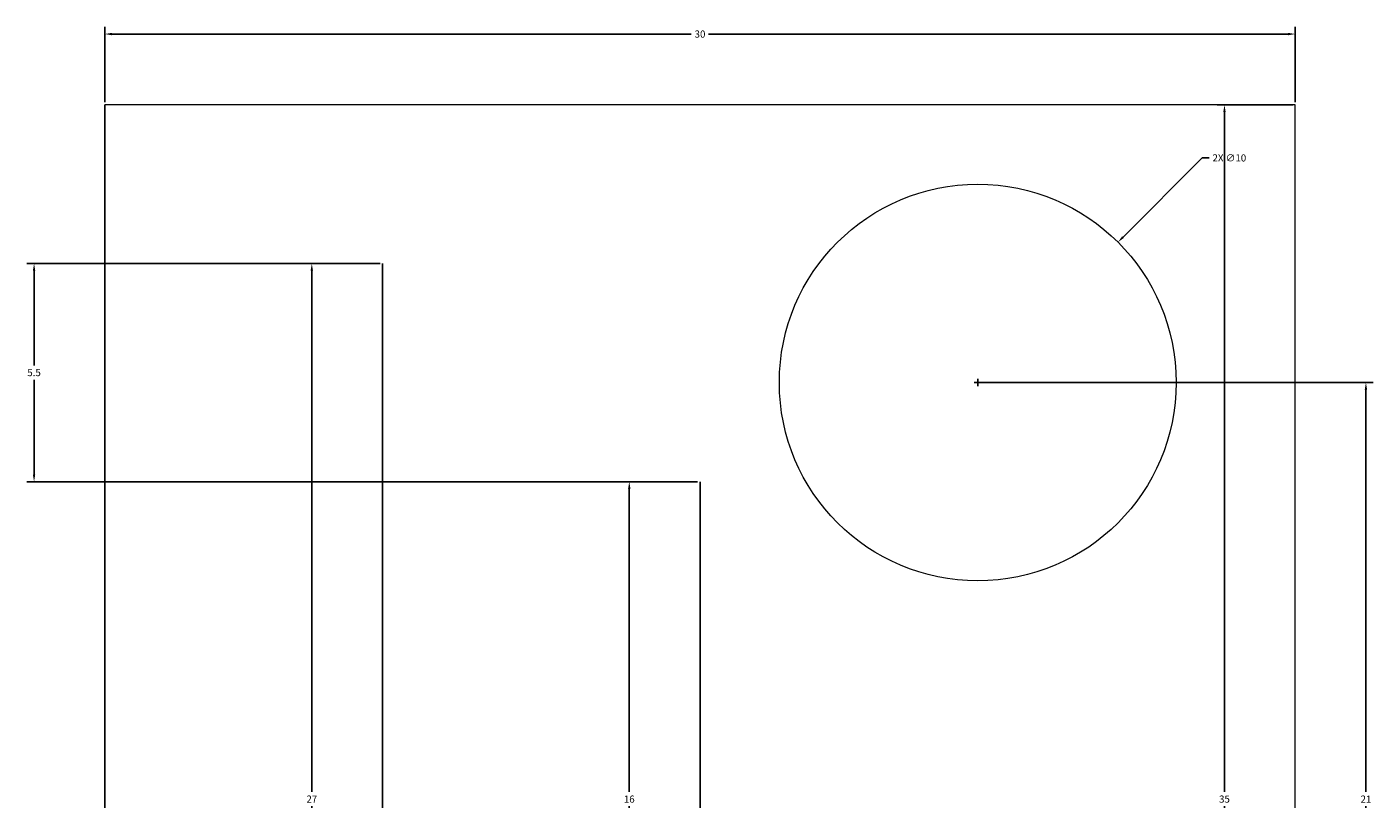
# Model space of a CAD drawing. Units: millimetres. Extents: x 136.9 to 170.9, y 96.9 to 135.8.
# Tile 2 of 2: x 136.9 to 170.9, y 116.3 to 135.8. Entities that reach past the tile are written whole.
import ezdxf

# ---------------------------------------------------------------- set-up
doc = ezdxf.new("R2010")
doc.units = ezdxf.units.MM
doc.layers.add('M-CONS', color=8, linetype='Continuous', lineweight=13)
doc.layers.add('M-DIMS', color=2, linetype='Continuous', lineweight=18)
doc.styles.get("Standard").update_dxf_attribs({"font": 'arial.ttf'})
doc.dimstyles.get("Standard").update_dxf_attribs({"dimtxt": 0.18, "dimasz": 0.18, "dimexe": 0.18, "dimexo": 0.0625, "dimgap": 0.09, "dimtad": 0, "dimtih": 1, "dimtoh": 1, "dimdec": 4, "dimzin": 0, "dimdsep": 46, "dimtxsty": 'Standard', "dimcen": 0.09, "dimadec": 0, "dimazin": 0, "dimtfac": 1, "dimtdec": 4, "dimtofl": 0, "dimtmove": 0, "dimatfit": 3, "dimfxl": 1, "dimtolj": 1, "dimtzin": 0, "dimarcsym": 0})

# ---------------------------------------------------------------- blocks, each defined once
blk = doc.blocks.new('*D1')
at = {"layer": 'Defpoints', "color": 0, "transparency": 16777216}
for p in [(168.89, 135.598), (138.89, 133.815), (168.89, 133.815)]:
    blk.add_point(p, dxfattribs=at)
at = {"layer": 'M-DIMS', "color": 0, "lineweight": -2, "transparency": 16777216}
for p, q in [((138.89, 133.878), (138.89, 135.778)), ((168.89, 133.878), (168.89, 135.778)), ((139.07, 135.598), (153.671, 135.598)), ((168.71, 135.598), (154.108, 135.598))]:
    blk.add_line(p, q, dxfattribs=at)
at = {"layer": 'M-DIMS', "color": 0, "transparency": 16777216}
for points in [[(139.07, 135.628), (139.07, 135.568), (138.89, 135.598)], [(168.71, 135.628), (168.71, 135.568), (168.89, 135.598)]]:
    blk.add_solid(points, dxfattribs=at)
at = {"layer": 'M-DIMS', "color": 0, "transparency": 16777216, "insert": (153.89, 135.598), "char_height": 0.18, "attachment_point": 5}
blk.add_mtext('\\A1;30', dxfattribs=at)
blk = doc.blocks.new('*D2')
at = {"layer": 'Defpoints', "color": 0, "transparency": 16777216}
for p in [(167.107, 133.815), (168.89, 133.815), (168.89, 98.815)]:
    blk.add_point(p, dxfattribs=at)
at = {"layer": 'M-DIMS', "color": 0, "lineweight": -2, "transparency": 16777216}
for p, q in [((168.827, 133.815), (166.927, 133.815)), ((167.107, 133.635), (167.107, 116.497)), ((167.107, 98.995), (167.107, 116.133)), ((168.827, 98.815), (166.927, 98.815))]:
    blk.add_line(p, q, dxfattribs=at)
at = {"layer": 'M-DIMS', "color": 0, "transparency": 16777216}
for points in [[(167.077, 133.635), (167.137, 133.635), (167.107, 133.815)], [(167.077, 98.995), (167.137, 98.995), (167.107, 98.815)]]:
    blk.add_solid(points, dxfattribs=at)
at = {"layer": 'M-DIMS', "color": 0, "transparency": 16777216, "insert": (167.107, 116.315), "char_height": 0.18, "attachment_point": 5}
blk.add_mtext('\\A1;35', dxfattribs=at)
blk = doc.blocks.new('*D7')
at = {"layer": 'Defpoints', "color": 0, "transparency": 16777216}
for p in [(144.107, 129.815), (145.89, 129.815), (145.89, 102.816)]:
    blk.add_point(p, dxfattribs=at)
at = {"layer": 'M-DIMS', "color": 0, "lineweight": -2, "transparency": 16777216}
for p, q in [((145.827, 129.815), (143.927, 129.815)), ((144.107, 129.635), (144.107, 116.496)), ((144.107, 102.996), (144.107, 116.135)), ((145.827, 102.816), (143.927, 102.816))]:
    blk.add_line(p, q, dxfattribs=at)
at = {"layer": 'M-DIMS', "color": 0, "transparency": 16777216}
for points in [[(144.077, 129.635), (144.137, 129.635), (144.107, 129.815)], [(144.077, 102.996), (144.137, 102.996), (144.107, 102.816)]]:
    blk.add_solid(points, dxfattribs=at)
at = {"layer": 'M-DIMS', "color": 0, "transparency": 16777216, "insert": (144.107, 116.315), "char_height": 0.18, "attachment_point": 5}
blk.add_mtext('\\A1;27', dxfattribs=at)
blk = doc.blocks.new('*D8')
at = {"layer": 'Defpoints', "color": 0, "transparency": 16777216}
for p in [(152.107, 124.315), (153.89, 124.315), (153.89, 108.315)]:
    blk.add_point(p, dxfattribs=at)
at = {"layer": 'M-DIMS', "color": 0, "lineweight": -2, "transparency": 16777216}
for p, q in [((153.827, 124.315), (151.927, 124.315)), ((152.107, 124.135), (152.107, 116.497)), ((152.107, 108.495), (152.107, 116.133)), ((153.827, 108.315), (151.927, 108.315))]:
    blk.add_line(p, q, dxfattribs=at)
at = {"layer": 'M-DIMS', "color": 0, "transparency": 16777216}
for points in [[(152.077, 124.135), (152.137, 124.135), (152.107, 124.315)], [(152.077, 108.495), (152.137, 108.495), (152.107, 108.315)]]:
    blk.add_solid(points, dxfattribs=at)
at = {"layer": 'M-DIMS', "color": 0, "transparency": 16777216, "insert": (152.107, 116.315), "char_height": 0.18, "attachment_point": 5}
blk.add_mtext('\\A1;16', dxfattribs=at)
blk = doc.blocks.new('*D9')
at = {"layer": 'Defpoints', "color": 0, "transparency": 16777216}
for p in [(145.89, 129.815), (137.107, 124.315), (153.89, 124.315)]:
    blk.add_point(p, dxfattribs=at)
at = {"layer": 'M-DIMS', "color": 0, "lineweight": -2, "transparency": 16777216}
for p, q in [((145.827, 129.815), (136.927, 129.815)), ((137.107, 129.635), (137.107, 127.247)), ((137.107, 124.495), (137.107, 126.884)), ((153.827, 124.315), (136.927, 124.315))]:
    blk.add_line(p, q, dxfattribs=at)
at = {"layer": 'M-DIMS', "color": 0, "transparency": 16777216}
for points in [[(137.077, 129.635), (137.137, 129.635), (137.107, 129.815)], [(137.077, 124.495), (137.137, 124.495), (137.107, 124.315)]]:
    blk.add_solid(points, dxfattribs=at)
at = {"layer": 'M-DIMS', "color": 0, "transparency": 16777216, "insert": (137.107, 127.065), "char_height": 0.18, "attachment_point": 5}
blk.add_mtext('\\A1;5.5', dxfattribs=at)
blk = doc.blocks.new('*D11')
at = {"layer": 'Defpoints', "color": 0, "transparency": 16777216}
for p in [(160.89, 126.815), (170.672, 126.815), (160.89, 105.815)]:
    blk.add_point(p, dxfattribs=at)
at = {"layer": 'M-DIMS', "color": 0, "lineweight": -2, "transparency": 16777216}
for p, q in [((160.952, 126.815), (170.852, 126.815)), ((170.672, 126.635), (170.672, 116.496)), ((170.672, 105.995), (170.672, 116.135)), ((160.952, 105.815), (170.852, 105.815))]:
    blk.add_line(p, q, dxfattribs=at)
at = {"layer": 'M-DIMS', "color": 0, "transparency": 16777216}
for points in [[(170.642, 126.635), (170.702, 126.635), (170.672, 126.815)], [(170.642, 105.995), (170.702, 105.995), (170.672, 105.815)]]:
    blk.add_solid(points, dxfattribs=at)
at = {"layer": 'M-DIMS', "color": 0, "transparency": 16777216, "insert": (170.672, 116.315), "char_height": 0.18, "attachment_point": 5}
blk.add_mtext('\\A1;21', dxfattribs=at)
blk = doc.blocks.new('*D12')
at = {"layer": 'Defpoints', "color": 0, "transparency": 16777216}
for p in [(164.423, 130.353), (157.356, 123.278)]:
    blk.add_point(p, dxfattribs=at)
at = {"layer": 'M-DIMS', "color": 0, "lineweight": -2, "transparency": 16777216}
for p, q in [((166.543, 132.476), (164.55, 130.48)), ((166.723, 132.476), (166.543, 132.476)), ((160.89, 126.725), (160.89, 126.905)), ((160.8, 126.815), (160.98, 126.815))]:
    blk.add_line(p, q, dxfattribs=at)
at = {"layer": 'M-DIMS', "color": 0, "transparency": 16777216}
blk.add_solid([(164.529, 130.502), (164.571, 130.459), (164.423, 130.353)], dxfattribs=at)
at = {"layer": 'M-DIMS', "color": 0, "transparency": 16777216, "insert": (167.23, 132.476), "char_height": 0.18, "attachment_point": 5}
blk.add_mtext('\\A1;2X ∅10', dxfattribs=at)

msp = doc.modelspace()

# ---------------------------------------------------------------- linework, layer by layer
at = {"layer": 'M-CONS'}
msp.add_lwpolyline([(168.89, 98.815), (168.89, 133.815), (138.89, 133.815), (138.89, 98.815)], close=True, dxfattribs=at)
at = {"layer": 'M-CONS', "extrusion": (1, -1e-16, 0), "elevation": 138.89}
msp.add_lwpolyline([(98.815, 55), (133.815, 55), (133.815, 0), (98.815, 0)], close=True, dxfattribs=at)
at = {"layer": 'M-CONS'}
msp.add_circle((160.89, 126.815), 5, dxfattribs=at)
at = {"layer": 'M-CONS', "extrusion": (1, -1e-16, 0)}
msp.add_circle((116.315, 18.918, 153.89), 8, dxfattribs=at)
at = {"layer": 'M-CONS', "extrusion": (1, 0, 1.7e-15)}
msp.add_rational_spline([(145.89, 113.315, 6.838), (145.89, 113.315, 3.419), (145.89, 113.315), (145.89, 114.815), (145.89, 116.315), (145.89, 117.815), (145.89, 119.315), (145.89, 119.315, 3.419), (145.89, 119.315, 6.838), (145.89, 131.08, 9.519), (145.89, 129.731, 21.509), (145.89, 128.382, 33.5), (145.89, 116.315, 33.5), (145.89, 104.249, 33.5), (145.89, 102.9, 21.509), (145.89, 101.551, 9.519), (145.89, 113.315, 6.838)], [1, 1, 1, 1, 1, 1, 1, 1, 1, 0.745591123387, 1, 0.745591123387, 1, 0.745591123387, 1, 0.745591123387, 1], degree=2, knots=[0, 0, 0, 1, 1, 2, 2, 3, 3, 4, 4, 5.45875, 5.45875, 6.9175, 6.9175, 8.376249, 8.376249, 9.834999, 9.834999, 9.834999], dxfattribs=at)

# ---------------------------------------------------------------- dimensions: what is measured, and where the dimension line sits
at = {"layer": 'M-DIMS'}
dim = msp.add_linear_dim(base=(168.89, 135.598), p1=(138.89, 133.815), p2=(168.89, 133.815), dimstyle='Standard', override={"dimdec": 0, "dimlfac": 1, "dimrnd": 0, "dimzin": 0, "dimdsep": 46, "dimlunit": 2}, dxfattribs=at)
dim.commit()
dim.dimension.update_dxf_attribs({"geometry": '*D1', "text_midpoint": (153.89, 135.598)})
for base, p1, p2, override, picture, middle in [((167.107, 133.815), (168.89, 98.815), (168.89, 133.815), {"dimdec": 0, "dimlfac": 1, "dimrnd": 0, "dimzin": 0, "dimdsep": 46, "dimlunit": 2}, '*D2', (167.107, 116.315)), ((137.107, 124.315), (145.89, 129.815), (153.89, 124.315), {"dimdec": 1, "dimlfac": 1, "dimrnd": 0, "dimzin": 0, "dimdsep": 46, "dimlunit": 2}, '*D9', (137.107, 127.065)), ((144.107, 129.815), (145.89, 102.816), (145.89, 129.815), {"dimdec": 0, "dimlfac": 1, "dimrnd": 0, "dimzin": 0, "dimdsep": 46, "dimlunit": 2}, '*D7', (144.107, 116.315)), ((170.672, 126.815), (160.89, 105.815), (160.89, 126.815), {"dimdec": 0, "dimlfac": 1, "dimrnd": 0, "dimzin": 0, "dimdsep": 46, "dimlunit": 2}, '*D11', (170.672, 116.315)), ((152.107, 124.315), (153.89, 108.315), (153.89, 124.315), {"dimdec": 0, "dimlfac": 1, "dimrnd": 0, "dimzin": 0, "dimdsep": 46, "dimlunit": 2}, '*D8', (152.107, 116.315))]:
    dim = msp.add_linear_dim(base=base, p1=p1, p2=p2, angle=90, dimstyle='Standard', override=override, dxfattribs=at)
    dim.commit()
    dim.dimension.update_dxf_attribs({"geometry": picture, "text_midpoint": middle})
dim = msp.add_diameter_dim_2p(p1=(157.356, 123.278), p2=(164.423, 130.353), text='2X <>', dimstyle='Standard', override={"dimdec": 0, "dimlfac": 1, "dimrnd": 0, "dimzin": 0, "dimdsep": 46, "dimlunit": 2}, dxfattribs=at)
dim.commit()
dim.dimension.update_dxf_attribs({"geometry": '*D12', "text_midpoint": (167.23, 132.476), "dimtype": 163})

doc.saveas('drawing.dxf')
